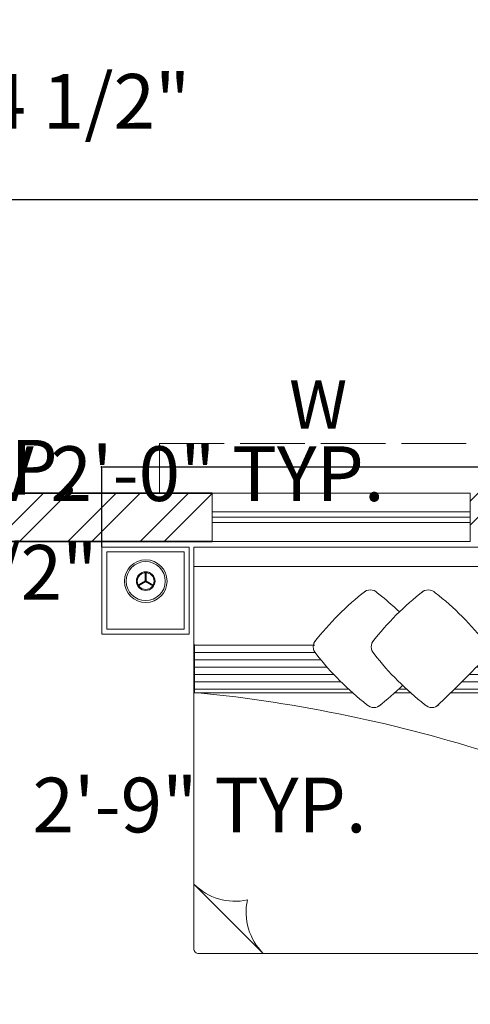
# Model space of a CAD drawing. Units: inches. Extents: x 2379 to 3013, y 1431 to 2110.
# Tile 9 of 10: x 2785 to 2869, y 1927 to 2110. Entities that reach past the tile are written whole.
import ezdxf

# ---------------------------------------------------------------- set-up
doc = ezdxf.new("R2010")
doc.units = ezdxf.units.IN
doc.linetypes.add('ACAD_ISO02W100', pattern=[15, 12, -3])
for name, color, linetype, lineweight in [('00 FURNITURE', 15, 'Continuous', 15), ('A-ANNO-DIMS', 2, 'Continuous', 18), ('A-ANNO-TEXT', 7, 'Continuous', 18), ('A-ROOF-OVHD', 11, 'ACAD_ISO02W100', 13), ('A-WALL-PATT', 8, 'Continuous', 13), ('WALL', 7, 'Continuous', 35), ('WINDOW', 4, 'Continuous', 15)]:
    doc.layers.add(name, color=color, linetype=linetype, lineweight=lineweight)
doc.styles.get("Standard").update_dxf_attribs({"font": 'arial.ttf'})
doc.dimstyles.get("Standard").update_dxf_attribs({"dimtxt": 10.18, "dimasz": 0.18, "dimexe": 0.18, "dimexo": 0.0625, "dimgap": 0.09, "dimtad": 0, "dimtih": 1, "dimtoh": 1, "dimdec": 0, "dimzin": 0, "dimdsep": 46, "dimlunit": 3, "dimtxsty": 'Standard', "dimcen": 0.09, "dimadec": 0, "dimazin": 0, "dimtfac": 1, "dimtdec": 0, "dimtofl": 0, "dimtmove": 0, "dimatfit": 3, "dimfxl": 1, "dimtolj": 1, "dimtzin": 0, "dimarcsym": 0})

# ---------------------------------------------------------------- blocks, each defined once
blk = doc.blocks.new('RGWTG')
at = {"layer": '00 FURNITURE'}
for p, q in [((578.23, 3473.51), (577.36, 3475.01)), ((578.36, 3473.58), (577.49, 3475.09)), ((578.23, 3473.58), (577.36, 3472.08)), ((578.36, 3473.51), (577.49, 3472)), ((578.29, 3473.62), (580.03, 3473.62)), ((578.29, 3473.47), (580.03, 3473.47)), ((521.93, 3464.58), (509.03, 3451.68)), ((509.03, 3422.63), (509.03, 3463.68)), ((509.93, 3464.58), (566.4, 3464.58)), ((557.53, 3463.84), (557.53, 3464.49)), ((557.53, 3464.49), (566.4, 3464.49)), ((558.2, 3464.49), (558.2, 3435.82)), ((559.57, 3464.49), (559.57, 3437.25)), ((560.94, 3464.49), (560.94, 3438.58)), ((562.3, 3464.49), (562.3, 3439.83)), ((563.67, 3464.49), (563.67, 3440.99)), ((565.04, 3464.49), (565.04, 3442.08)), ((566.4, 3464.58), (580.98, 3464.58)), ((566.4, 3464.49), (566.4, 3442.08)), ((566.4, 3464.49), (566.4, 3463.84)), ((580.98, 3464.58), (580.98, 3416.72)), ((558.2, 3426.48), (558.2, 3425.04)), ((509.03, 3400.68), (509.03, 3422.63)), ((558.2, 3416.13), (558.2, 3399.95)), ((580.98, 3416.72), (580.98, 3400.68)), ((559.57, 3414.75), (559.57, 3399.95)), ((560.94, 3413.39), (560.94, 3399.95)), ((562.3, 3412.04), (562.3, 3399.95)), ((563.67, 3410.72), (563.67, 3399.95)), ((580.08, 3399.78), (509.93, 3399.78)), ((557.53, 3399.95), (557.53, 3400.6)), ((566.4, 3399.95), (557.53, 3399.95)), ((566.4, 3400.6), (566.4, 3399.95)), ((578.23, 3390.78), (577.36, 3392.29)), ((578.36, 3390.86), (577.49, 3392.36)), ((578.23, 3390.86), (577.36, 3389.36)), ((578.36, 3390.78), (577.49, 3389.28)), ((578.29, 3390.9), (580.03, 3390.9)), ((578.29, 3390.74), (580.03, 3390.74))]:
    blk.add_line(p, q, dxfattribs=at)
for points in [[(568.43, 3465.48), (584.63, 3465.48), (584.63, 3481.68), (568.43, 3481.68)], [(569.33, 3466.38), (583.73, 3466.38), (583.73, 3480.78), (569.33, 3480.78)], [(580.98, 3399.78), (584.63, 3399.78), (584.63, 3464.58), (580.98, 3464.58)], [(568.43, 3398.88), (584.63, 3398.88), (584.63, 3382.68), (568.43, 3382.68)], [(569.33, 3397.98), (583.73, 3397.98), (583.73, 3383.58), (569.33, 3383.58)]]:
    blk.add_lwpolyline(points, close=True, dxfattribs=at)
for points in [[(566.52, 3464.49), (557.53, 3464.49), (557.53, 3435.08)], [(557.53, 3427.21), (557.53, 3424.3)], [(557.53, 3416.82), (557.53, 3399.95), (566.4, 3399.95), (566.4, 3409.94)]]:
    blk.add_lwpolyline(points, dxfattribs=at)
for centre, radius in [((578.29, 3473.54), 3.97), ((578.29, 3473.54), 3.63), ((578.29, 3473.54), 1.74), ((578.29, 3473.54), 1.56), ((578.29, 3390.82), 3.97), ((578.29, 3390.82), 3.63), ((578.29, 3390.82), 1.74), ((578.29, 3390.82), 1.56)]:
    blk.add_circle(centre, radius, dxfattribs=at)
for centre, radius, start, end in [((509.93, 3463.68), 0.9, 90, 180), ((529.65, 3456.88), 10.9, 135.0361, 191.9278), ((290.56, 3490.52), 268.3, 342.2214, 354.2925), ((516.73, 3443.97), 10.9, 78.0722, 134.9639), ((598.15, 3399.01), 54.32, 127.931, 142.069), ((566.05, 3440.57), 1.82, 45, 135), ((533.58, 3399.31), 54.32, 37.931, 52.069), ((556.59, 3431.11), 1.82, 135, 225), ((574.84, 3431.77), 1.82, 315, 45), ((597.87, 3463.6), 54.32, 217.931, 224.141), ((598.15, 3388.23), 54.32, 127.931, 142.069), ((566.05, 3429.78), 1.82, 45, 135), ((533.58, 3388.53), 54.32, 37.931, 52.069), ((533.28, 3463.88), 54.32, 316.32, 322.069), ((556.59, 3420.33), 1.82, 135, 225), ((574.84, 3420.99), 1.82, 315, 45), ((765.33, 3619.75), 290.45, 223.6069, 226.2326), ((533.28, 3453.1), 54.32, 307.931, 322.069), ((565.44, 3411.05), 1.47, 225.9674, 326.8337), ((545.02, 3395.29), 13.35, 20.4224, 85.5825), ((509.93, 3400.68), 0.9, 180, 270), ((580.08, 3400.68), 0.9, 270, 0)]:
    blk.add_arc(centre, radius, start, end, dxfattribs=at)
blk = doc.blocks.new('*D14')
at = {"layer": 'A-ANNO-DIMS', "color": 0, "lineweight": -2, "transparency": 16777216}
for p, q in [((2469.63, 2021.67), (2469.63, 2076.34)), ((2469.81, 2076.16), (2694.9, 2076.16)), ((2937.45, 2076.16), (2712.35, 2076.16)), ((2937.63, 2021.67), (2937.63, 2076.34))]:
    blk.add_line(p, q, dxfattribs=at)
at = {"layer": 'A-ANNO-DIMS', "color": 0, "transparency": 16777216}
for points in [[(2469.81, 2076.19), (2469.81, 2076.13), (2469.63, 2076.16)], [(2937.45, 2076.19), (2937.45, 2076.13), (2937.63, 2076.16)]]:
    blk.add_solid(points, dxfattribs=at)
at = {"layer": 'Defpoints', "color": 0, "transparency": 16777216}
for p in [(2937.63, 2076.16), (2469.63, 2021.61), (2937.63, 2021.61)]:
    blk.add_point(p, dxfattribs=at)
at = {"layer": 'A-ANNO-DIMS', "color": 0, "transparency": 16777216, "insert": (2703.63, 2076.16), "char_height": 10.18, "attachment_point": 5}
blk.add_mtext("\\A1;39'", dxfattribs=at)
blk = doc.blocks.new('WIN-48IN')
for p, q in [((0, 48), (0, 0)), ((9, 48), (0, 48)), ((3.5, 48), (3.5, 0)), ((4.5, 48), (4.5, 0)), ((5.5, 48), (5.5, 0)), ((9, 0), (9, 48)), ((9, 0), (0, 0))]:
    blk.add_line(p, q)
blk = doc.blocks.new('*D26')
at = {"layer": 'A-ANNO-DIMS', "color": 0, "lineweight": -2, "transparency": 16777216}
for p, q in [((2688.62, 1958.67), (2688.62, 1963.76)), ((2688.8, 1963.58), (2721.58, 1963.58)), ((2721.76, 1958.67), (2721.76, 1963.76)), ((2721.76, 1963.58), (2721.94, 1963.58))]:
    blk.add_line(p, q, dxfattribs=at)
at = {"layer": 'A-ANNO-DIMS', "color": 0, "transparency": 16777216}
for points in [[(2688.8, 1963.61), (2688.8, 1963.55), (2688.62, 1963.58)], [(2721.58, 1963.61), (2721.58, 1963.55), (2721.76, 1963.58)]]:
    blk.add_solid(points, dxfattribs=at)
at = {"layer": 'Defpoints', "color": 0, "transparency": 16777216}
for p in [(2721.76, 1963.58), (2688.62, 1958.61), (2721.76, 1958.61)]:
    blk.add_point(p, dxfattribs=at)
at = {"layer": 'A-ANNO-DIMS', "color": 0, "transparency": 16777216, "insert": (2787.18, 1963.58), "char_height": 10.18, "attachment_point": 5}
blk.add_mtext('\\A1;DOOR D1 2\'-9" TYP.', dxfattribs=at)
blk = doc.blocks.new('*D28')
at = {"layer": 'A-ANNO-DIMS', "color": 0, "lineweight": -2, "transparency": 16777216}
for p, q in [((2714.17, 2021.67), (2714.17, 2025.39)), ((2738.17, 2021.67), (2738.17, 2025.39)), ((2714.35, 2025.21), (2737.99, 2025.21)), ((2738.17, 2025.21), (2738.35, 2025.21))]:
    blk.add_line(p, q, dxfattribs=at)
at = {"layer": 'A-ANNO-DIMS', "color": 0, "transparency": 16777216}
for points in [[(2714.35, 2025.24), (2714.35, 2025.18), (2714.17, 2025.21)], [(2737.99, 2025.24), (2737.99, 2025.18), (2738.17, 2025.21)]]:
    blk.add_solid(points, dxfattribs=at)
at = {"layer": 'Defpoints', "color": 0, "transparency": 16777216}
for p in [(2738.17, 2025.21), (2714.17, 2021.61), (2738.17, 2021.61)]:
    blk.add_point(p, dxfattribs=at)
at = {"layer": 'A-ANNO-DIMS', "color": 0, "transparency": 16777216, "insert": (2797.39, 2025.21), "char_height": 10.18, "attachment_point": 5}
blk.add_mtext('\\A1;VENT V 2\'-0" TYP.', dxfattribs=at)
blk = doc.blocks.new('*D30')
at = {"layer": 'A-ANNO-DIMS', "color": 0, "lineweight": -2, "transparency": 16777216}
for p, q in [((2800.26, 2026.41), (2800.08, 2026.41)), ((2800.26, 2011.63), (2800.26, 2026.59)), ((2899.08, 2026.41), (2800.44, 2026.41)), ((2899.26, 2011.63), (2899.26, 2026.59))]:
    blk.add_line(p, q, dxfattribs=at)
at = {"layer": 'A-ANNO-DIMS', "color": 0, "transparency": 16777216}
for points in [[(2800.44, 2026.44), (2800.44, 2026.38), (2800.26, 2026.41)], [(2899.08, 2026.44), (2899.08, 2026.38), (2899.26, 2026.41)]]:
    blk.add_solid(points, dxfattribs=at)
at = {"layer": 'Defpoints', "color": 0, "transparency": 16777216}
for p in [(2800.26, 2026.41), (2800.26, 2011.56), (2899.26, 2011.56)]:
    blk.add_point(p, dxfattribs=at)
at = {"layer": 'A-ANNO-DIMS', "color": 0, "transparency": 16777216, "insert": (2724.54, 2026.41), "char_height": 10.18, "attachment_point": 5}
blk.add_mtext('\\A1;BED GROUP 8\'-3" TYP.', dxfattribs=at)
blk = doc.blocks.new('*D46')
at = {"layer": 'A-ANNO-DIMS', "color": 0, "lineweight": -2, "transparency": 16777216}
for p, q in [((2736.09, 2012.61), (2737.93, 2012.61)), ((2737.75, 2012.43), (2737.75, 2012.2)), ((2736.09, 2001.09), (2737.93, 2001.09)), ((2737.75, 2001.27), (2737.75, 2001.49))]:
    blk.add_line(p, q, dxfattribs=at)
at = {"layer": 'A-ANNO-DIMS', "color": 0, "transparency": 16777216}
for points in [[(2737.72, 2012.43), (2737.78, 2012.43), (2737.75, 2012.61)], [(2737.72, 2001.27), (2737.78, 2001.27), (2737.75, 2001.09)]]:
    blk.add_solid(points, dxfattribs=at)
at = {"layer": 'Defpoints', "color": 0, "transparency": 16777216}
for p in [(2736.02, 2012.61), (2737.75, 2012.61), (2736.02, 2001.09)]:
    blk.add_point(p, dxfattribs=at)
at = {"layer": 'A-ANNO-DIMS', "color": 0, "transparency": 16777216, "insert": (2737.75, 2006.85), "char_height": 10.18, "attachment_point": 5}
blk.add_mtext('\\A1;SHOWER 0\'-11 1/2"', dxfattribs=at)
blk = doc.blocks.new('*D65')
at = {"layer": 'A-ANNO-DIMS', "color": 0, "lineweight": -2, "transparency": 16777216}
for p, q in [((2735.32, 1920.86), (2735.32, 2094.64)), ((2735.5, 2094.46), (2763.45, 2094.46)), ((2763.63, 1924.67), (2763.63, 2094.64)), ((2763.63, 2094.46), (2763.81, 2094.46))]:
    blk.add_line(p, q, dxfattribs=at)
at = {"layer": 'A-ANNO-DIMS', "color": 0, "transparency": 16777216}
for points in [[(2735.5, 2094.49), (2735.5, 2094.43), (2735.32, 2094.46)], [(2763.45, 2094.49), (2763.45, 2094.43), (2763.63, 2094.46)]]:
    blk.add_solid(points, dxfattribs=at)
at = {"layer": 'Defpoints', "color": 0, "transparency": 16777216}
for p in [(2763.63, 2094.46), (2763.63, 1924.61), (2735.32, 1920.79)]:
    blk.add_point(p, dxfattribs=at)
at = {"layer": 'A-ANNO-DIMS', "color": 0, "transparency": 16777216, "insert": (2789.38, 2094.46), "char_height": 10.18, "attachment_point": 5}
blk.add_mtext('\\A1;2\'-4 1/2"', dxfattribs=at)
blk = doc.blocks.new('*D66')
at = {"layer": 'A-ANNO-DIMS', "color": 0, "lineweight": -2, "transparency": 16777216}
for p, q in [((2980.62, 1924.61), (2980.62, 1924.79)), ((2980.62, 1924.79), (2980.8, 1924.79)), ((2763.69, 1924.61), (2980.8, 1924.61)), ((2980.62, 1920.97), (2980.62, 1924.43)), ((2735.39, 1920.79), (2980.8, 1920.79))]:
    blk.add_line(p, q, dxfattribs=at)
at = {"layer": 'A-ANNO-DIMS', "color": 0, "transparency": 16777216}
for points in [[(2980.59, 1924.43), (2980.65, 1924.43), (2980.62, 1924.61)], [(2980.59, 1920.97), (2980.65, 1920.97), (2980.62, 1920.79)]]:
    blk.add_solid(points, dxfattribs=at)
at = {"layer": 'Defpoints', "color": 0, "transparency": 16777216}
for p in [(2763.63, 1924.61), (2980.62, 1924.61), (2735.32, 1920.79)]:
    blk.add_point(p, dxfattribs=at)
at = {"layer": 'A-ANNO-DIMS', "color": 0, "transparency": 16777216, "insert": (2994.42, 1924.79), "char_height": 10.18, "attachment_point": 5}
blk.add_mtext('\\A1;0\'-4"', dxfattribs=at)

msp = doc.modelspace()

# ---------------------------------------------------------------- hatches: boundary and pattern name
at = {"layer": 'A-WALL-PATT'}
h = msp.add_hatch(dxfattribs=at)
h.set_pattern_fill('ANSI32', color=256)
h.paths.add_polyline_path([(2925.63, 1862.61), (2815.63, 1862.61), (2815.63, 1858.61), (2827.63, 1858.61), (2827.63, 1810.61), (2815.63, 1810.61), (2815.63, 1806.61), (2850.78, 1806.61), (2850.78, 1810.61), (2831.63, 1810.61), (2831.63, 1858.61), (2925.63, 1858.61)])
h.paths.add_polyline_path([(2925.63, 1810.61), (2880.78, 1810.61), (2880.78, 1806.61), (2925.63, 1806.61)], flags=17)
h.paths.add_polyline_path([(2633.75, 1660.61), (2594.63, 1660.61), (2481.63, 1660.61), (2481.63, 1651.61), (2588.63, 1651.61), (2588.63, 1570.61), (2624.28, 1570.61), (2624.28, 1574.61), (2592.63, 1574.61), (2592.63, 1651.61), (2633.75, 1651.61)])
h.paths.add_polyline_path([(2594.63, 1809.61), (2481.63, 1809.61), (2481.63, 1805.61), (2594.63, 1805.61)])
h.paths.add_polyline_path([(2594.63, 2012.61), (2597.21, 2012.61), (2597.21, 2021.61), (2588.21, 2021.61), (2588.21, 2012.61), (2590.63, 2012.61), (2590.63, 1845.61), (2594.63, 1845.61)])
h.paths.add_polyline_path([(2767.63, 2012.61), (2770.27, 2012.61), (2770.27, 2021.61), (2761.27, 2021.61), (2761.27, 2012.61), (2763.63, 2012.61), (2763.63, 1928.61), (2691.63, 1928.61), (2643.63, 1928.61), (2643.63, 1924.61), (2691.63, 1924.61), (2763.63, 1924.61), (2763.63, 1858.61), (2779.63, 1858.61), (2779.63, 1862.61), (2767.63, 1862.61)])
h.paths.add_polyline_path([(2613.63, 2012.61), (2613.63, 2021.61), (2597.21, 2021.61), (2597.21, 2012.61)])
h.paths.add_polyline_path([(2508.33, 2012.61), (2508.33, 2021.61), (2478.63, 2021.61), (2478.63, 2012.61)])
h.paths.add_polyline_path([(2556.33, 2021.61), (2556.33, 2012.61), (2588.21, 2012.61), (2588.21, 2021.61)])
h.paths.add_polyline_path([(2659.15, 2012.61), (2659.15, 2021.61), (2643.63, 2021.61), (2643.63, 1958.61), (2661.63, 1958.61), (2661.63, 1962.61), (2647.63, 1962.61), (2647.63, 2012.61)])
h.paths.add_polyline_path([(2714.17, 2012.61), (2714.17, 2021.61), (2683.15, 2021.61), (2683.15, 2012.61), (2691.63, 2012.61), (2691.63, 1958.61), (2695.63, 1958.61), (2695.63, 2012.61)])
h.paths.add_polyline_path([(2738.17, 2021.61), (2738.17, 2012.61), (2761.27, 2012.61), (2761.27, 2021.61)])
h.paths.add_polyline_path([(2820.76, 2012.61), (2820.76, 2021.61), (2770.27, 2021.61), (2770.27, 2012.61)])
h.paths.add_polyline_path([(2868.76, 2021.61), (2868.76, 2012.61), (2928.63, 2012.61), (2928.63, 2021.61)])
h.paths.add_polyline_path([(2928.63, 1962.9), (2937.63, 1962.9), (2937.63, 2009.61), (2928.63, 2009.61)])
h.paths.add_polyline_path([(2937.63, 1914.9), (2928.63, 1914.9), (2928.63, 1863.8), (2937.63, 1863.8)])
h.paths.add_polyline_path([(2928.63, 1846.59), (2937.63, 1846.59), (2937.63, 1854.8), (2928.63, 1854.8)])
h.paths.add_polyline_path([(2937.63, 1822.59), (2928.63, 1822.59), (2928.63, 1813.62), (2937.63, 1813.62)])
h.paths.add_polyline_path([(2928.63, 1778.48), (2937.63, 1778.48), (2937.63, 1813.62), (2928.63, 1813.62), (2928.63, 1810.61), (2925.63, 1810.61), (2925.63, 1806.61), (2928.63, 1806.61)])
h.paths.add_polyline_path([(2816.22, 1651.61), (2816.22, 1660.61), (2767.63, 1660.61), (2767.63, 1806.61), (2779.63, 1806.61), (2779.63, 1810.61), (2763.63, 1810.61), (2763.63, 1660.61), (2688.63, 1660.61), (2688.63, 1810.61), (2684.63, 1810.61), (2684.63, 1660.61), (2669.75, 1660.61), (2669.75, 1651.61), (2763.63, 1651.61), (2763.63, 1574.61), (2672.28, 1574.61), (2672.28, 1570.61), (2767.63, 1570.61), (2767.63, 1651.61)])
h.paths.add_polyline_path([(2864.22, 1660.61), (2864.22, 1651.61), (2937.63, 1651.61), (2937.63, 1730.48), (2928.63, 1730.48), (2928.63, 1660.61)])
h.paths.add_polyline_path([(2469.63, 1975.19), (2478.63, 1975.19), (2478.63, 2009.61), (2469.63, 2009.61)])
h.paths.add_polyline_path([(2478.63, 1927.19), (2469.63, 1927.19), (2469.63, 1811.02), (2478.63, 1811.02)])
h.paths.add_polyline_path([(2469.63, 1758.04), (2478.63, 1758.04), (2478.63, 1802.02), (2469.63, 1802.02)])
h.paths.add_polyline_path([(2478.63, 1710.04), (2469.63, 1710.04), (2469.63, 1660.61), (2478.63, 1660.61)])

# ---------------------------------------------------------------- linework, layer by layer
at = {"layer": 'A-ROOF-OVHD'}
for p, q in [((2810.99, 2021.61), (2810.99, 2030.79)), ((2810.99, 2030.79), (2879.94, 2030.79))]:
    msp.add_line(p, q, dxfattribs=at)
at = {"layer": 'WALL'}
for p, q in [((2738.17, 2021.61), (2820.76, 2021.61)), ((2767.63, 2012.61), (2820.76, 2012.61))]:
    msp.add_line(p, q, dxfattribs=at)

# ---------------------------------------------------------------- block references
at = {"layer": '00 FURNITURE', "rotation": 89.99999999999999}
msp.add_blockref('RGWTG', (6281.94, 1426.94), dxfattribs=at)
at = {"layer": 'WINDOW', "rotation": 269.9999985709198}
msp.add_blockref('WIN-48IN', (2820.76, 2021.61), dxfattribs=at)

# ---------------------------------------------------------------- texts
at = {"layer": 'A-ANNO-TEXT', "insert": (2835.08, 2042.55), "char_height": 9, "attachment_point": 1}
msp.add_mtext_dynamic_manual_height_columns('W', width=106.8919, gutter_width=12.5, heights=[0], dxfattribs=at)

# ---------------------------------------------------------------- dimensions: what is measured, and where the dimension line sits
at = {"layer": 'A-ANNO-DIMS'}
for base, p1, p2, override, picture, middle in [((2763.63, 2094.46), (2735.32, 1920.79), (2763.63, 1924.61), {"dimdec": 1, "dimlfac": 1, "dimrnd": 0, "dimzin": 1, "dimdsep": 46, "dimlunit": 4, "dimfrac": 2}, '*D65', (2789.38, 2094.46)), ((2937.63, 2076.16), (2469.63, 2021.61), (2937.63, 2021.61), {"dimclrd": 0, "dimclre": 0, "dimclrt": 0}, '*D14', (2703.63, 2076.16))]:
    dim = msp.add_linear_dim(base=base, p1=p1, p2=p2, dimstyle='Standard', override=override, dxfattribs=at)
    dim.commit()
    dim.dimension.update_dxf_attribs({"geometry": picture, "text_midpoint": middle})
for base, p1, p2, angle, text, picture, middle in [((2800.26, 2026.41), (2899.26, 2011.56), (2800.26, 2011.56), 180, 'BED GROUP <> TYP.', '*D30', (2724.54, 2026.41)), ((2737.75, 2012.61), (2736.02, 2001.09), (2736.02, 2012.61), 90, 'SHOWER <>', '*D46', (2737.75, 2006.85))]:
    dim = msp.add_linear_dim(base=base, p1=p1, p2=p2, angle=angle, text=text, dimstyle='Standard', override={"dimdec": 1, "dimlfac": 1, "dimrnd": 0, "dimzin": 1, "dimdsep": 46, "dimlunit": 4, "dimfrac": 2}, dxfattribs=at)
    dim.commit()
    dim.dimension.update_dxf_attribs({"geometry": picture, "text_midpoint": middle})
for base, p1, p2, text, picture, middle in [((2738.17, 2025.21), (2714.17, 2021.61), (2738.17, 2021.61), 'VENT V <> TYP.', '*D28', (2797.39, 2025.21)), ((2721.76, 1963.58), (2688.62, 1958.61), (2721.76, 1958.61), 'DOOR D1 <> TYP.', '*D26', (2787.18, 1963.58))]:
    dim = msp.add_linear_dim(base=base, p1=p1, p2=p2, text=text, dimstyle='Standard', override={"dimdec": 1, "dimlfac": 1, "dimrnd": 0, "dimzin": 1, "dimdsep": 46, "dimlunit": 4, "dimfrac": 2}, dxfattribs=at)
    dim.commit()
    dim.dimension.update_dxf_attribs({"geometry": picture, "text_midpoint": middle})
dim = msp.add_linear_dim(base=(2980.62, 1924.61), p1=(2735.32, 1920.79), p2=(2763.63, 1924.61), angle=90, dimstyle='Standard', override={"dimdec": 1, "dimlfac": 1, "dimrnd": 0, "dimzin": 1, "dimdsep": 46, "dimlunit": 4, "dimfrac": 2}, dxfattribs=at)
dim.commit()
dim.dimension.update_dxf_attribs({"geometry": '*D66', "text_midpoint": (2994.42, 1924.79)})

doc.saveas('drawing.dxf')
